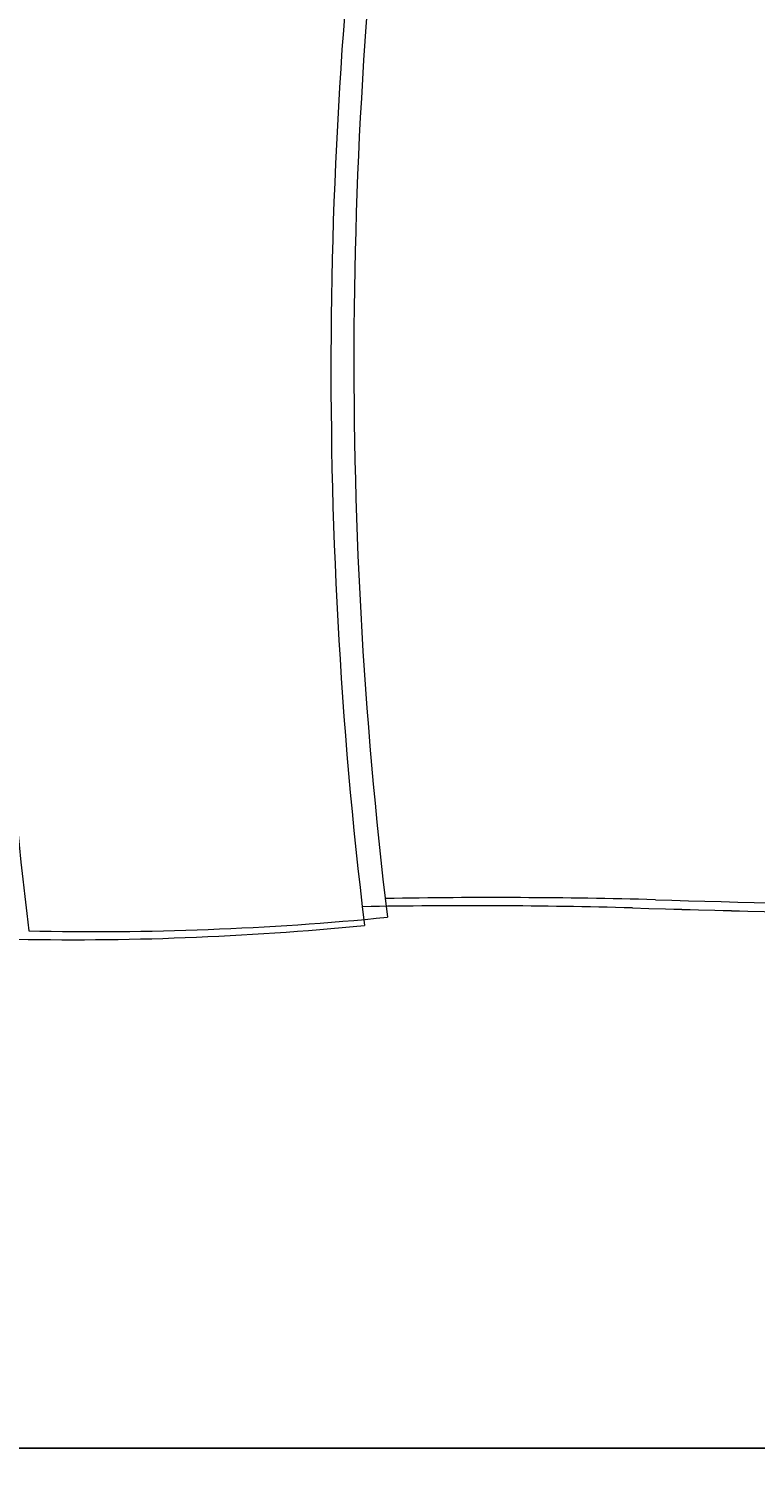
# Model space of a CAD drawing. Units: inches. Extents: x 2168 to 3056, y 1130 to 2629.
# Tile 26 of 42: x 2485 to 2505, y 2307 to 2347. Entities that reach past the tile are written whole.
import ezdxf

# ---------------------------------------------------------------- set-up
doc = ezdxf.new("R2010")
doc.units = ezdxf.units.IN
doc.layers.add('A-ANNO-DIMS', color=2, linetype='Continuous', lineweight=18)
doc.layers.add('A-FURN', color=8, linetype='Continuous', lineweight=13)
doc.styles.get("Standard").update_dxf_attribs({"font": 'arial.ttf'})
doc.dimstyles.get("Standard").update_dxf_attribs({"dimtxt": 0.18, "dimasz": 0.18, "dimexe": 0.18, "dimexo": 0.0625, "dimgap": 0.09, "dimtad": 0, "dimtih": 1, "dimtoh": 1, "dimdec": 4, "dimzin": 0, "dimdsep": 46, "dimtxsty": 'Standard', "dimcen": 0.09, "dimadec": 0, "dimazin": 0, "dimtfac": 1, "dimtdec": 4, "dimtofl": 0, "dimtmove": 0, "dimatfit": 3, "dimfxl": 1, "dimtolj": 1, "dimtzin": 0, "dimarcsym": 0})

# ---------------------------------------------------------------- blocks, each defined once
blk = doc.blocks.new('BED-DOUBLE')
for centre, radius, start, end in [((156.956, 17.984), 129.02, 171.78449, 186.90062), ((156.956, 17.984), 129.02, 171.78449, 186.90062), ((156.317, 17.756), 129.02, 171.78449, 186.90062), ((156.317, 17.756), 129.02, 171.78449, 186.90062), ((182.692, 21.587), 164.969, 176.08655, 186.78213), ((31.174, -167.307), 170.11, 88.4762, 91.00819), ((31.174, -167.307), 170.11, 88.4762, 91.00819), ((31.813, -167.079), 170.11, 88.4762, 91.00819), ((31.813, -167.079), 170.11, 88.4762, 91.00819), ((51.253, 485.051), 482.31, 268.22771, 271.71854), ((51.253, 485.051), 482.31, 268.22771, 271.71854), ((20.736, 85.39), 83.306, 268.72178, 275.60397), ((20.736, 85.39), 83.306, 268.72178, 275.60397), ((50.614, 484.823), 482.31, 268.22771, 271.71854), ((50.614, 484.822), 482.31, 268.22771, 271.71854), ((20.097, 85.162), 83.306, 268.72178, 275.60397), ((20.097, 85.162), 83.306, 268.72178, 275.60397)]:
    blk.add_arc(centre, radius, start, end)
blk = doc.blocks.new('*D14')
at = {"layer": 'A-ANNO-DIMS', "color": 0, "lineweight": -2, "transparency": 16777216}
for p, q in [((2466.224, 2319.873), (2466.224, 2307.523)), ((2547.772, 2319.873), (2547.772, 2307.523)), ((2466.404, 2307.703), (2506.18, 2307.703)), ((2547.592, 2307.703), (2507.815, 2307.703))]:
    blk.add_line(p, q, dxfattribs=at)
at = {"layer": 'A-ANNO-DIMS', "color": 0, "transparency": 16777216}
for points in [[(2466.404, 2307.733), (2466.404, 2307.673), (2466.224, 2307.703)], [(2547.592, 2307.733), (2547.592, 2307.673), (2547.772, 2307.703)]]:
    blk.add_solid(points, dxfattribs=at)
at = {"layer": 'Defpoints', "color": 0, "transparency": 16777216}
for p in [(2466.224, 2319.935), (2547.772, 2319.935), (2547.772, 2307.703)]:
    blk.add_point(p, dxfattribs=at)
at = {"layer": 'A-ANNO-DIMS', "color": 0, "transparency": 16777216, "insert": (2506.998, 2307.703), "char_height": 0.18, "attachment_point": 5}
blk.add_mtext('\\A1;BED 82 TYP.', dxfattribs=at)

msp = doc.modelspace()

# ---------------------------------------------------------------- block references
at = {"layer": 'A-FURN'}
msp.add_blockref('BED-DOUBLE', (2466.223, 2320.021), dxfattribs=at)

# ---------------------------------------------------------------- dimensions: what is measured, and where the dimension line sits
at = {"layer": 'A-ANNO-DIMS'}
dim = msp.add_linear_dim(base=(2547.772, 2307.703), p1=(2466.224, 2319.935), p2=(2547.772, 2319.935), text='BED <> TYP.', dimstyle='Standard', override={"dimdec": 0, "dimlfac": 1, "dimrnd": 0, "dimzin": 0, "dimdsep": 46, "dimlunit": 2}, dxfattribs=at)
dim.commit()
dim.dimension.update_dxf_attribs({"geometry": '*D14', "text_midpoint": (2506.998, 2307.703)})

doc.saveas('drawing.dxf')
